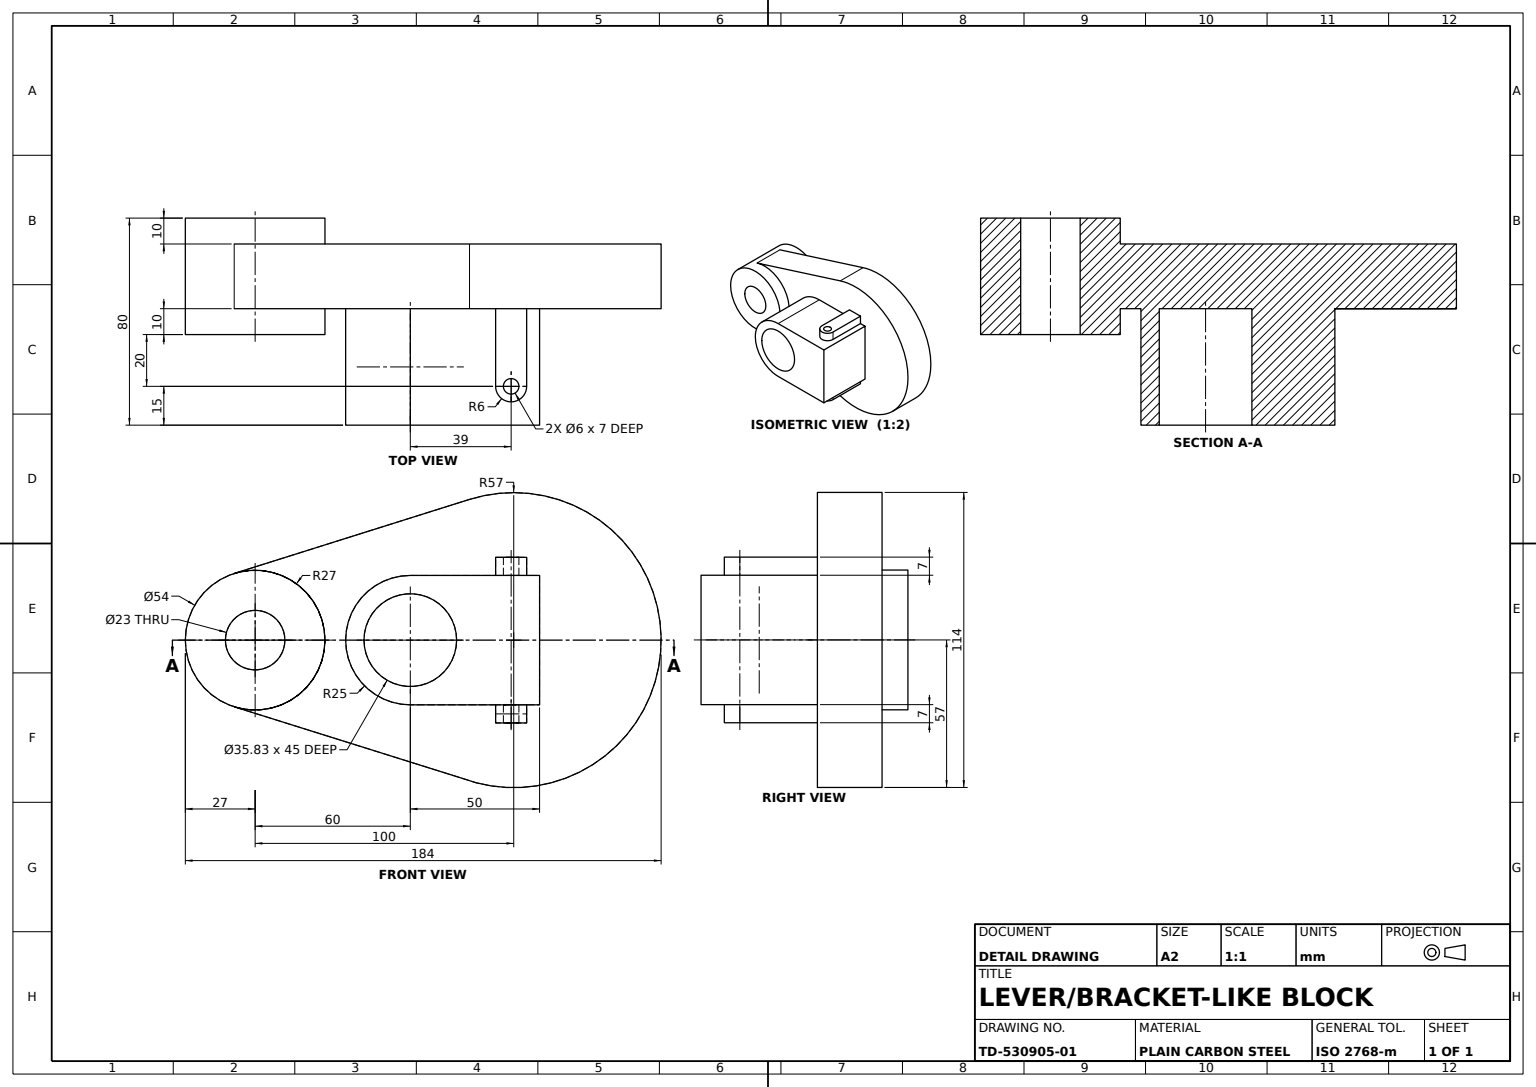
from build123d import *

# Parameters (mm, degrees)
BASE_PLATE_DEPTH      = 25
FRONT_HUB_SKETCH_R    = 27
FRONT_HUB_54_DEPTH    = 10
REAR_START            = 10
REAR_HUB_SKETCH_R     = 27
REAR_HUB_54_DEPTH     = 10
HUB_BORE_SKETCH_R     = 11.5
HUB_BORE_23_DEPTH     = 50
BEARING_BLOCK_DEPTH   = 45
BLOCK_BORE_SKETCH_R   = 17.912737299
BLOCK_BORE_35_8_DEPTH = 45
LUG_TAB_1_DEPTH       = 7
LUG_START             = 7
LUG_TAB_2_DEPTH       = 7
LUG_HOLE_1_SKETCH_R   = 3
LUG_HOLE_1_6_DEPTH    = 7
LUG_START_2           = -7
LUG_HOLE_2_SKETCH_R   = 3
LUG_HOLE_2_6_DEPTH    = 7


with BuildPart() as part:
    # Base Plate Sketch → Base Plate (new body)
    with BuildSketch(Plane.XY):
        with BuildLine():
            Line((-17.1, 54.374534481), (-108.1, 25.756358438))
            ThreePointArc((-108.1, 25.756358438), (-127, 0), (-108.1, -25.756358438))
            Line((-108.1, -25.756358438), (-108.05082408, -25.771771993))
            Line((-108.05082408, -25.771771993), (-20.094170087, -53.340644245))
            ThreePointArc((-20.094170087, -53.340644245), (56.977991401, -1.583823185), (-17.1, 54.374534481))
        make_face()
    extrude(amount=BASE_PLATE_DEPTH)

    # Front Hub Sketch → Front Hub _54 (add)
    with BuildSketch(Plane.XY.offset(25)):
        with Locations(Location((-100, 0, 0), (0, 0, 252.542396876))):
            Circle(FRONT_HUB_SKETCH_R)
    extrude(amount=FRONT_HUB_54_DEPTH)

    # Rear Hub Sketch → Rear Hub _54 (add)
    with BuildSketch(Plane(origin=(0, 0, 0), x_dir=(-1, 0, 0), z_dir=(0, 0, -1)).offset(REAR_START)):
        with Locations((100, 0)):
            Circle(REAR_HUB_SKETCH_R)
    extrude(amount=-REAR_HUB_54_DEPTH)

    # Hub Bore Sketch → Hub Bore _23 (cut)
    with BuildSketch(Plane.XY.offset(35)):
        with Locations((-100, 0)):
            Circle(HUB_BORE_SKETCH_R)
    extrude(amount=-HUB_BORE_23_DEPTH, mode=Mode.SUBTRACT)

    # Bearing Block Sketch → Bearing Block (add)
    with BuildSketch(Plane.XY.offset(25)):
        with BuildLine():
            Line((-40, 25), (10, 25))
            Line((10, 25), (10, -25))
            Line((10, -25), (-40, -25))
            ThreePointArc((-40, -25), (-65, 0), (-40, 25))
        make_face()
    extrude(amount=BEARING_BLOCK_DEPTH)

    # Block Bore Sketch → Block Bore _35.8 (cut)
    with BuildSketch(Plane.XY.offset(70)):
        with Locations((-40, 0)):
            Circle(BLOCK_BORE_SKETCH_R)
    extrude(amount=-BLOCK_BORE_35_8_DEPTH, mode=Mode.SUBTRACT)

    # Lug Tab 1 Sketch → Lug Tab 1 (add)
    with BuildSketch(Plane.XZ.offset(25)):
        with BuildLine():
            Line((5, 25), (5, 55))
            ThreePointArc((5, 55), (-1, 61), (-7, 55))
            Line((-7, 55), (-7, 25))
            Line((-7, 25), (5, 25))
        make_face()
    extrude(amount=LUG_TAB_1_DEPTH)

    # Lug Tab 2 Sketch → Lug Tab 2 (add)
    with BuildSketch(Plane(origin=(0, 25, 0), x_dir=(1, 0, 0), z_dir=(0, 1, 0)).offset(LUG_START)):
        with BuildLine():
            Line((5, -25), (5, -55))
            ThreePointArc((5, -55), (-1, -61), (-7, -55))
            Line((-7, -55), (-7, -25))
            Line((-7, -25), (5, -25))
        make_face()
    extrude(amount=-LUG_TAB_2_DEPTH)

    # Lug Hole 1 Sketch → Lug Hole 1 _6 (cut)
    with BuildSketch(Plane.XZ.offset(32)):
        with Locations(Location((-1, 55, 0), (0, 0, 270))):
            Circle(LUG_HOLE_1_SKETCH_R)
    extrude(amount=-LUG_HOLE_1_6_DEPTH, mode=Mode.SUBTRACT)

    # Lug Hole 2 Sketch → Lug Hole 2 _6 (cut)
    with BuildSketch(Plane(origin=(0, 32, 0), x_dir=(1, 0, 0), z_dir=(0, 1, 0)).offset(LUG_START_2)):
        with Locations(Location((-1, -55, 0), (0, 0, 90))):
            Circle(LUG_HOLE_2_SKETCH_R)
    extrude(amount=LUG_HOLE_2_6_DEPTH, mode=Mode.SUBTRACT)


solid = part.part
